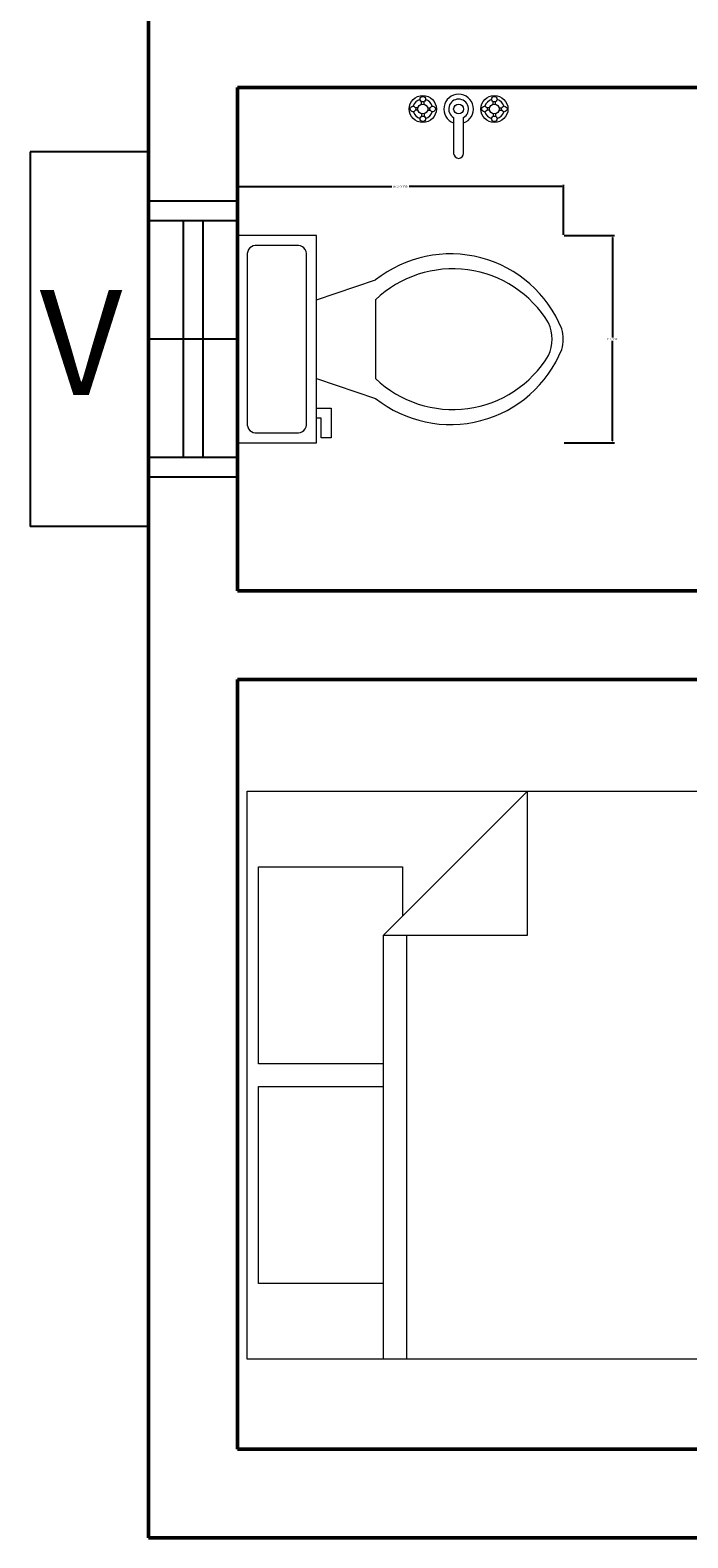
# Model space of a CAD drawing. Units: inches. Extents: x -105 to 1196, y -792 to 119.
# Tile 2 of 23: x -57 to 9, y -438 to -285. Entities that reach past the tile are written whole.
import ezdxf

# ---------------------------------------------------------------- set-up
doc = ezdxf.new("R2010")
doc.units = ezdxf.units.IN
doc.header["$MEASUREMENT"] = 0
for name, color, linetype, lineweight in [('A-ANNO-DIMS', 2, 'Continuous', 18), ('A-ANNO-TEXT', 7, 'Continuous', 25), ('A-FLOR-FIXT', 8, 'Continuous', 18), ('A-FURN', 8, 'Continuous', 18), ('A-GLAZ', 4, 'Continuous', 25), ('A-WALL', 3, 'Continuous', 50)]:
    doc.layers.add(name, color=color, linetype=linetype, lineweight=lineweight)
doc.styles.get("Standard").update_dxf_attribs({"font": 'arial.ttf'})
doc.dimstyles.get("Standard").update_dxf_attribs({"dimtxt": 0.18, "dimasz": 0.18, "dimexe": 0.18, "dimexo": 0.0625, "dimgap": 0.09, "dimtad": 0, "dimtih": 1, "dimtoh": 1, "dimdec": 1, "dimzin": 0, "dimdsep": 46, "dimlunit": 4, "dimtxsty": 'Standard', "dimcen": 0.09, "dimadec": 0, "dimazin": 0, "dimtfac": 1, "dimtdec": 1, "dimtofl": 0, "dimtmove": 0, "dimatfit": 3, "dimfxl": 1, "dimtolj": 1, "dimtzin": 0, "dimarcsym": 0})

# ---------------------------------------------------------------- blocks, each defined once
blk = doc.blocks.new('Toilet - top')
for p, q in [((9.5, -6), (9.5, -2)), ((-10, -8.5), (-8, -8.5)), ((-10, -9.5), (-10, -8.5)), ((-8, -8.5), (-8, -8)), ((-7, -8), (-7, -9.5)), ((-4, -8), (-6, -14)), ((4, -8), (6, -14)), ((-7, -9.5), (-10, -9.5)), ((4, -14), (-4, -14))]:
    blk.add_line(p, q)
blk.add_lwpolyline([(10.5, -8), (10.5, 0), (-10.5, 0), (-10.5, -8)], close=True)
for points in [[(8.5, -1), (-8.5, -1)], [(-9.5, -2), (-9.5, -6)], [(-8.5, -7), (8.5, -7)]]:
    blk.add_lwpolyline(points)
for centre, radius, start, end in [((-8.62, -1.88), 0.884, 81.8699, 188.1301), ((8.62, -1.88), 0.884, 351.8699, 98.1301), ((-8.62, -6.12), 0.884, 171.8699, 278.1301), ((8.62, -6.12), 0.884, 261.8699, 8.1301), ((3.52, -21.58), 12.17, 141.4691, 247.9714), ((4.2, -21.82), 11.33, 136.3677, 238.9468), ((-3.52, -21.58), 12.17, 292.0284, 38.5307), ((-4.2, -21.82), 11.33, 301.053, 43.6321), ((0, -27.88), 4, 245.7318, 294.2682), ((0, -29), 4, 254.8605, 285.1395)]:
    blk.add_arc(centre, radius, start, end)
blk = doc.blocks.new('Faucet - Bathroom top')
for p, q in [((-4.107, 0.125), (-4.375, 0.125)), ((-3.75, 0.4788), (-3.75, 0.75)), ((-3.5, 0.482), (-3.5, 0.75)), ((-3.1461, 0.125), (-2.875, 0.125)), ((3.143, 0.125), (2.875, 0.125)), ((3.5, 0.4788), (3.5, 0.75)), ((3.75, 0.482), (3.75, 0.75)), ((4.1039, 0.125), (4.375, 0.125)), ((-4.1039, -0.125), (-4.375, -0.125)), ((-3.75, -0.4821), (-3.75, -0.75)), ((-3.5, -0.4789), (-3.5, -0.75)), ((-3.143, -0.125), (-2.875, -0.125)), ((-0.5, -0.8639), (-0.5, -4.5)), ((0.5, -4.5), (0.5, -0.8631)), ((3.1461, -0.125), (2.875, -0.125)), ((3.5, -0.4821), (3.5, -0.75)), ((3.75, -0.4789), (3.75, -0.75)), ((4.107, -0.125), (4.375, -0.125))]:
    blk.add_line(p, q)
for centre, radius in [((-3.625, 0), 1.375), ((-4.625, 0), 0.2795), ((-3.625, 0), 0.5), ((-3.625, 1), 0.2795), ((-2.625, 0), 0.2795), ((0, 0), 0.5), ((3.625, 0), 1.375), ((2.625, 0), 0.2795), ((3.625, 0), 0.5), ((3.625, 1), 0.2795), ((4.625, 0), 0.2795), ((-3.625, -1), 0.2795), ((3.625, -1), 0.2795)]:
    blk.add_circle(centre, radius)
for centre, radius, start, end in [((-3.625, 0), 1, 105.2407, 164.2093), ((-3.625, 0), 1, 16.44125, 74.07887), ((0, 0), 1.5, 289.6514, 250.3603), ((0, 0), 1, 300.3431, 239.7554), ((3.625, 0), 1, 106.12, 164.0884), ((3.625, 0), 1, 16.23422, 73.90469), ((-3.625, 0), 1, 196.2342, 253.9047), ((-3.625, 0), 1, 286.12, 344.0884), ((3.625, 0), 1, 196.4413, 254.0789), ((3.625, 0), 1, 285.2407, 344.2093), ((0, -4.5), 0.5, 180, 0)]:
    blk.add_arc(centre, radius, start, end)
blk = doc.blocks.new('Bed - Queen')
for p, q in [((0, -80.00003), (0, 0)), ((0, 0), (59.99999, 0)), ((59.99999, 0), (59.99999, -80.00003)), ((7.99999, -1.2), (28.79998, -1.2)), ((7.99999, -14.4), (7.99999, -1.2)), ((28.79998, -1.2), (28.79998, -14.4)), ((31.19999, -1.2), (51.99999, -1.2)), ((31.19999, -14.4), (31.19999, -1.2)), ((51.99999, -1.2), (51.99999, -16.4)), ((0, -14.4), (44.8, -14.4)), ((59.99999, -29.6), (44.8, -14.4)), ((44.8, -14.4), (44.8, -29.6)), ((44.8, -16.8), (0, -16.8)), ((51.99999, -16.4), (46.79936, -16.4)), ((44.8, -29.6), (59.99999, -29.6)), ((59.99999, -80.00003), (0, -80.00003))]:
    blk.add_line(p, q)
blk = doc.blocks.new('VENT-600')
for p, q in [((0, 9), (0, 21)), ((38, 21), (0, 21)), ((38, 9), (38, 21)), ((5, 9), (0, 9)), ((5, 0), (5, 9)), ((33, 0), (33, 9)), ((33, 9), (38, 9))]:
    blk.add_line(p, q)
blk = doc.blocks.new('*D61')
at = {"layer": 'A-ANNO-DIMS', "color": 0, "lineweight": -2, "transparency": 16777216}
for p, q in [((-36.26, -306.16), (-36.26, -301.09)), ((-36.08, -301.27), (-20.62, -301.27)), ((-3.39, -301.27), (-18.85, -301.27)), ((-3.21, -306.16), (-3.21, -301.09))]:
    blk.add_line(p, q, dxfattribs=at)
at = {"layer": 'A-ANNO-DIMS', "color": 0, "transparency": 16777216}
for points in [[(-36.08, -301.24), (-36.08, -301.3), (-36.26, -301.27)], [(-3.39, -301.24), (-3.39, -301.3), (-3.21, -301.27)]]:
    blk.add_solid(points, dxfattribs=at)
at = {"layer": 'Defpoints', "color": 0, "transparency": 16777216}
for p in [(-36.26, -301.27), (-36.26, -306.23), (-3.21, -306.23)]:
    blk.add_point(p, dxfattribs=at)
at = {"layer": 'A-ANNO-DIMS', "color": 0, "transparency": 16777216, "insert": (-19.73, -301.27), "char_height": 0.18, "attachment_point": 5}
blk.add_mtext('\\A1;WC 2\'-9" TYP.', dxfattribs=at)
blk = doc.blocks.new('*D62')
at = {"layer": 'A-ANNO-DIMS', "color": 0, "lineweight": -2, "transparency": 16777216}
for p, q in [((-3.15, -306.23), (1.93, -306.23)), ((1.75, -306.41), (1.75, -316.55)), ((1.75, -327.05), (1.75, -316.91)), ((-3.15, -327.23), (1.93, -327.23))]:
    blk.add_line(p, q, dxfattribs=at)
at = {"layer": 'A-ANNO-DIMS', "color": 0, "transparency": 16777216}
for points in [[(1.72, -306.41), (1.78, -306.41), (1.75, -306.23)], [(1.72, -327.05), (1.78, -327.05), (1.75, -327.23)]]:
    blk.add_solid(points, dxfattribs=at)
at = {"layer": 'Defpoints', "color": 0, "transparency": 16777216}
for p in [(-3.21, -306.23), (1.75, -306.23), (-3.21, -327.23)]:
    blk.add_point(p, dxfattribs=at)
at = {"layer": 'A-ANNO-DIMS', "color": 0, "transparency": 16777216, "insert": (1.75, -316.73), "char_height": 0.18, "attachment_point": 5}
blk.add_mtext('\\A1;1\'-9" TYP.', dxfattribs=at)

msp = doc.modelspace()

# ---------------------------------------------------------------- linework, layer by layer
at = {"layer": 'A-GLAZ'}
for p, q in [((-36.26, -304.73), (-45.26, -304.73)), ((-41.76, -304.73), (-41.76, -328.73)), ((-39.76, -304.73), (-39.76, -328.73)), ((-36.26, -316.73), (-45.26, -316.73)), ((-36.26, -328.73), (-45.26, -328.73))]:
    msp.add_line(p, q, dxfattribs=at)
at = {"layer": 'A-WALL'}
for p, q in [((-45.26, -125.23), (-45.26, -291.23)), ((-45.26, -291.23), (-45.26, -438.23)), ((-36.26, -291.23), (59.74, -291.23)), ((-36.26, -291.23), (-36.26, -342.23)), ((-36.26, -291.23), (-36.26, -342.23)), ((-36.26, -342.23), (68.74, -342.23)), ((-36.26, -351.23), (68.74, -351.23)), ((-36.26, -351.23), (-36.26, -429.23)), ((-36.26, -429.23), (120.74, -429.23)), ((-45.26, -438.23), (129.74, -438.23))]:
    msp.add_line(p, q, dxfattribs=at)

# ---------------------------------------------------------------- block references
at = {"layer": 'A-FLOR-FIXT'}
msp.add_blockref('Faucet - Bathroom top', (-13.85, -293.4), dxfattribs=at)
at = {"layer": 'A-FLOR-FIXT', "rotation": 90}
msp.add_blockref('Toilet - top', (-36.26, -316.73), dxfattribs=at)
at = {"layer": 'A-FURN', "xscale": 0.9593862173514477, "yscale": 0.9593862173514477, "zscale": 0.9593862173514477, "rotation": 90}
msp.add_blockref('Bed - Queen', (-35.26, -420.11), dxfattribs=at)
at = {"layer": 'A-GLAZ', "rotation": 90.00000000000006}
msp.add_blockref('VENT-600', (-36.26, -335.73), dxfattribs=at)

# ---------------------------------------------------------------- texts
at = {"layer": 'A-ANNO-TEXT'}
msp.add_text('V', height=10.64, dxfattribs=at).set_placement((-56.28, -322.4))

# ---------------------------------------------------------------- dimensions: what is measured, and where the dimension line sits
at = {"layer": 'A-ANNO-DIMS'}
for base, p1, p2, angle, text, picture, middle in [((-36.2556, -301.2705), (-3.2094, -306.2275), (-36.2556, -306.2275), 180, 'WC <> TYP.', '*D61', (-19.7325, -301.2705)), ((1.75, -306.23), (-3.21, -327.23), (-3.21, -306.23), 90, '<> TYP.', '*D62', (1.75, -316.73))]:
    dim = msp.add_linear_dim(base=base, p1=p1, p2=p2, angle=angle, text=text, dimstyle='Standard', override={"dimdec": 1, "dimlfac": 1, "dimrnd": 0, "dimzin": 1, "dimdsep": 46, "dimlunit": 4, "dimfrac": 2}, dxfattribs=at)
    dim.commit()
    dim.dimension.update_dxf_attribs({"geometry": picture, "text_midpoint": middle})

doc.saveas('drawing.dxf')
